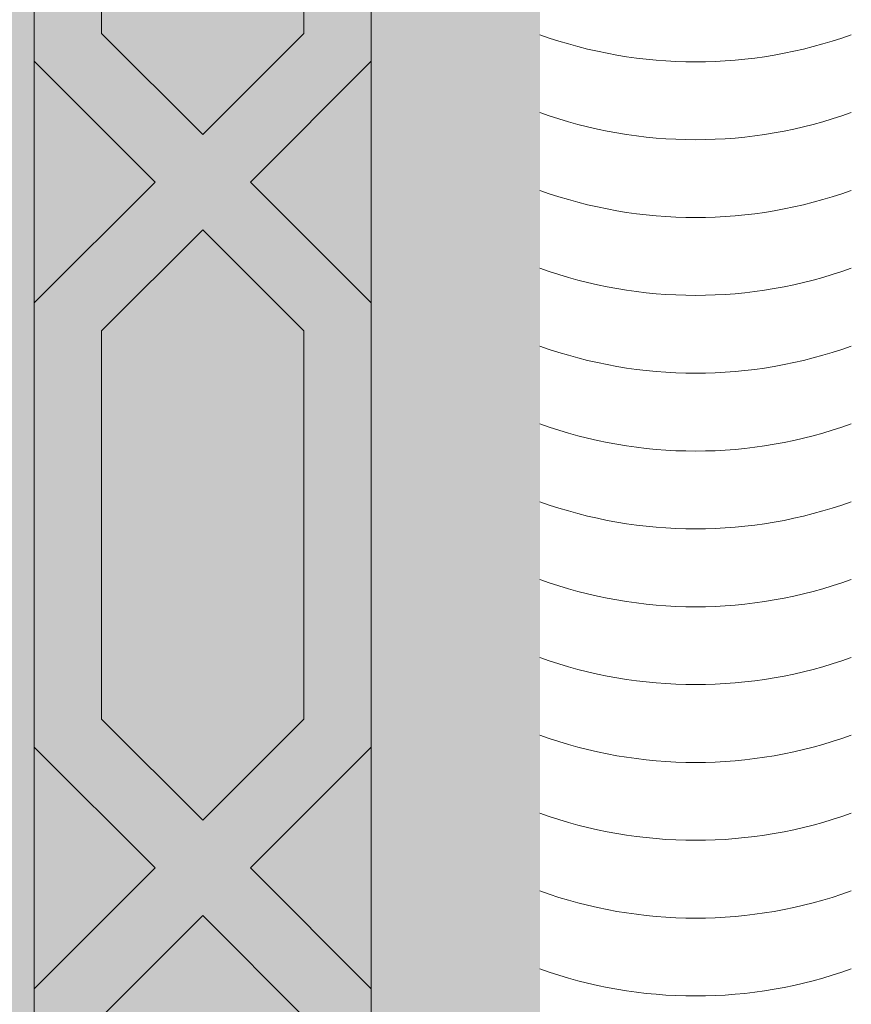
# Model space of a CAD drawing. Units: inches. Extents: x 844 to 2234, y 346 to 1084.
# Tile 39 of 93: x 1262.421 to 1265.567, y 701.353 to 705.079. Entities that reach past the tile are written whole.
import ezdxf

# ---------------------------------------------------------------- set-up
doc = ezdxf.new("R2010")
doc.units = ezdxf.units.IN
doc.header["$MEASUREMENT"] = 0
doc.layers.add('furniture', color=8, linetype='Continuous', lineweight=18)
doc.layers.add('RA-AP-01$0$INT', color=35, linetype='Continuous', lineweight=5)
doc.layers.add('RA-AP-01$0$FURN', color=3, linetype='Continuous')

# ---------------------------------------------------------------- blocks, each defined once
blk = doc.blocks.new('A$C18D01794')
at = {"layer": 'RA-AP-01$0$INT'}
h = blk.add_hatch(color=256, dxfattribs=at)
h.paths.add_polyline_path([(4.355206456958071, -6.156712009588037), (4.355206456958071, -8.056712009588038), (5.455206456958072, -8.056712009588038), (5.455206456958072, -6.156712009588037)])
h.paths.add_polyline_path([(4.405206456958072, -8.006712009588039), (4.405206456958072, -6.206712009588038), (5.405206456958072, -6.206712009588038), (5.405206456958072, -8.006712009588039)], flags=16)
h = blk.add_hatch(color=256, dxfattribs=at)
h.paths.add_polyline_path([(4.505206456958071, -7.585498806127123), (4.46934859260189, -7.549640941759413), (4.505206456958071, -7.513783077414768), (4.505206456958071, -7.381963272220687), (4.469348592616735, -7.346105407867824), (4.505206456958071, -7.310247543514964), (4.505206456958071, -7.178427738324996), (4.469348592586679, -7.142569873965138), (4.505206456952245, -7.106712009588038), (4.476922185709333, -7.106712009588038), (4.455206456960671, -7.128427738343681), (4.433490728198047, -7.106712009588038), (4.405206456946033, -7.106712009588036), (4.441064321339216, -7.142569873969684), (4.40520645695807, -7.178427738362358), (4.405206456958072, -7.310247543472698), (4.441064321364728, -7.346105407867826), (4.40520645695807, -7.381963272262947), (4.40520645695807, -7.513783077378263), (4.441064321354429, -7.549640941786153), (4.405206456958072, -7.585498806170974), (4.405206456958072, -7.717318611286652), (4.441064321333084, -7.753176475673194), (4.405206456958072, -7.789034340036673), (4.405206456958072, -8.006712009588039), (4.644348592588106, -8.006712009588039), (4.680206456964639, -7.970854145211967), (4.716064321341165, -8.006712009588039), (4.869348592586113, -8.006712009588039), (4.905206456964143, -7.970854145210465), (4.941064321342174, -8.006712009588039), (5.094348592587118, -8.006712009588037), (5.130206456963649, -7.970854145211967), (5.166064321340178, -8.006712009588039), (5.405206456958072, -8.006712009588039), (5.405206456958072, -7.789034340024526), (5.369348592595202, -7.753176475673196), (5.40520645695807, -7.717318611298797), (5.40520645695807, -7.585498806158829), (5.369348592573859, -7.549640941786151), (5.40520645695807, -7.51378307739041), (5.40520645695807, -7.381963272250803), (5.36934859256356, -7.346105407867824), (5.405206456958072, -7.310247543484846), (5.405206456958072, -7.178427738350217), (5.369348592589068, -7.142569873969682), (5.405206456982249, -7.106712009588038), (5.376922185730244, -7.106712009588038), (5.355206456967613, -7.128427738343679), (5.333490728218955, -7.10671200958804), (5.305206456976043, -7.106712009588042), (5.341064321341609, -7.142569873965136), (5.305206456958072, -7.178427738337141), (5.305206456958072, -7.310247543502816), (5.34106432131155, -7.346105407867824), (5.305206456958072, -7.381963272232832), (5.30520645695807, -7.513783077402624), (5.341064321326395, -7.549640941759413), (5.305206456958072, -7.585498806139263), (5.305206456958072, -7.717318611299605), (5.341064321347738, -7.753176475677737), (5.305206456958072, -7.78903434007894), (5.30520645695807, -7.906712009588039), (5.166064321336834, -7.906712009588039), (5.130206456963647, -7.942569873961684), (5.094348592590464, -7.906712009588039), (4.941064321338827, -7.906712009588041), (4.905206456964145, -7.942569873963183), (4.869348592589459, -7.906712009588039), (4.716064321337822, -7.906712009588041), (4.680206456964641, -7.942569873961684), (4.644348592591453, -7.906712009588039), (4.505206456958071, -7.906712009588039), (4.505206456958071, -7.789034340066795), (4.469348592580545, -7.753176475677738), (4.505206456958071, -7.717318611311748)])
h.paths.add_polyline_path([(4.485206456974132, -7.709034340046354), (4.45520645695909, -7.739034340051736), (4.425206456974128, -7.709034340057131), (4.425206456993394, -7.593783077384998), (4.45520645699153, -7.563783077396511), (4.485206456993396, -7.593783077408017)], flags=16)
h.paths.add_polyline_path([(4.455206456954537, -7.767318611299197), (4.485206456958242, -7.797318611312542), (4.48520645695951, -7.912569873958716), (4.45520645695415, -7.942569873954422), (4.425206456957888, -7.912569873967813), (4.425206456957888, -7.797318611286197)], flags=16)
h.paths.add_polyline_path([(4.455206456964794, -7.535498806149051), (4.42520645696469, -7.5054988061393), (4.425206456983954, -7.390247543486406), (4.455206456990734, -7.360247543489279), (4.485206456983953, -7.39024754349214), (4.485206456964687, -7.505498806158811)], flags=16)
h.paths.add_polyline_path([(4.499348592588947, -7.926712009585049), (4.636064321340932, -7.926712009585049), (4.666064321342317, -7.956712009586821), (4.636064321343707, -7.986712009585048), (4.499348592575121, -7.986712009585048), (4.469348592591685, -7.956712009591957)], flags=16)
h.paths.add_polyline_path([(4.425206456957888, -7.940854145195974), (4.471064321332215, -7.986712009585049), (4.425206456957888, -7.986712009585049)], flags=16)
h.paths.add_polyline_path([(4.455206456990734, -7.331963272246367), (4.425206456989053, -7.301963272254337), (4.425206456969784, -7.186712009596224), (4.455206456965226, -7.156712009591144), (4.485206456969787, -7.186712009586051), (4.485206456989053, -7.301963272238404)], flags=16)
h.paths.add_polyline_path([(4.72434859258714, -7.926712009586255), (4.861064321340141, -7.926712009586248), (4.891064321340324, -7.956712009586823), (4.861064321340513, -7.986712009586252), (4.724348592586768, -7.986712009586252), (4.694348592586956, -7.956712009586821)], flags=16)
h.paths.add_polyline_path([(4.919348592587961, -7.956712009586821), (4.949348592588145, -7.92671200958625), (5.08606432134115, -7.926712009586253), (5.116064321341327, -7.956712009586823), (5.086064321341519, -7.986712009586252), (4.949348592587774, -7.986712009586252)], flags=16)
h.paths.add_polyline_path([(5.144348592585967, -7.956712009586823), (5.174348592587358, -7.926712009585049), (5.311064321339338, -7.926712009585049), (5.3410643213366, -7.956712009591957), (5.311064321353163, -7.986712009585048), (5.174348592584576, -7.986712009585048)], flags=16)
h.paths.add_polyline_path([(5.32520645693489, -7.593783077408021), (5.355206456936755, -7.563783077396511), (5.385206456934894, -7.593783077384998), (5.38520645695416, -7.709034340057128), (5.355206456969194, -7.739034340051736), (5.325206456954153, -7.709034340046352)], flags=16)
h.paths.add_polyline_path([(5.325206456970042, -7.797318611312542), (5.355206456973747, -7.767318611299197), (5.385206456970398, -7.7973186112862), (5.385206456970398, -7.912569873967816), (5.355206456974136, -7.942569873954422), (5.325206456968778, -7.912569873958716)], flags=16)
h.paths.add_polyline_path([(5.325206456963599, -7.505498806158811), (5.325206456944333, -7.39024754349214), (5.355206456937552, -7.360247543489279), (5.385206456944332, -7.39024754348641), (5.385206456963596, -7.505498806139303), (5.355206456963492, -7.53549880614905)], flags=16)
h.paths.add_polyline_path([(5.32520645693923, -7.301963272238403), (5.3252064569585, -7.186712009586051), (5.355206456963062, -7.156712009591142), (5.3852064569585, -7.186712009596224), (5.385206456939234, -7.301963272254338), (5.355206456937552, -7.331963272246369)], flags=16)
h.paths.add_polyline_path([(5.339348592596071, -7.986712009585048), (5.385206456970398, -7.940854145195972), (5.385206456970396, -7.986712009585048)], flags=16)
h = blk.add_hatch(color=256, dxfattribs=at)
h.paths.add_polyline_path([(4.469348592586677, -7.142569873965136), (4.505206456958073, -7.178427738324996), (4.505206456958071, -7.106712009582215)])
h.paths.add_polyline_path([(4.455206456960671, -7.128427738343681), (4.476922185709333, -7.106712009588038), (4.433490728198045, -7.106712009588038)])
h.paths.add_polyline_path([(4.405206456958073, -7.178427738362358), (4.441064321339218, -7.142569873969684), (4.40520645695807, -7.106712009600073)])
h.paths.add_polyline_path([(4.425206456989053, -7.301963272254335), (4.455206456990736, -7.331963272246371), (4.485206456989055, -7.301963272238399), (4.48520645696979, -7.186712009586054), (4.455206456965227, -7.15671200959114), (4.425206456969784, -7.186712009596224)])
h.paths.add_polyline_path([(4.505206456958073, -7.381963272220689), (4.505206456958071, -7.310247543514961), (4.469348592616738, -7.346105407867826)])
h.paths.add_polyline_path([(4.425206456964688, -7.5054988061393), (4.455206456964794, -7.535498806149051), (4.485206456964689, -7.505498806158811), (4.485206456983951, -7.390247543492138), (4.455206456990736, -7.360247543489277), (4.425206456983956, -7.39024754348641)])
h.paths.add_polyline_path([(4.425206456974126, -7.709034340057128), (4.455206456959092, -7.739034340051736), (4.485206456974132, -7.709034340046356), (4.485206456993396, -7.593783077408017), (4.45520645699153, -7.563783077396511), (4.425206456993394, -7.593783077384999)])
h.paths.add_polyline_path([(4.46934859260189, -7.549640941759415), (4.505206456958071, -7.585498806127123), (4.505206456958073, -7.513783077414766)])
h.paths.add_polyline_path([(4.405206456958073, -7.585498806170972), (4.441064321354427, -7.549640941786151), (4.405206456958072, -7.513783077378263)])
h.paths.add_polyline_path([(4.405206456958072, -7.789034340036673), (4.441064321333084, -7.753176475673194), (4.405206456958072, -7.71731861128665)])
h.paths.add_polyline_path([(4.469348592580547, -7.75317647567774), (4.505206456958071, -7.789034340066795), (4.505206456958071, -7.717318611311744)])
h.paths.add_polyline_path([(4.425206456957888, -7.912569873967814), (4.45520645695415, -7.942569873954422), (4.485206456959507, -7.912569873958718), (4.48520645695824, -7.797318611312542), (4.455206456954537, -7.767318611299197), (4.425206456957888, -7.797318611286202)])
h.paths.add_polyline_path([(4.425206456957888, -7.986712009585049), (4.471064321332215, -7.986712009585049), (4.425206456957888, -7.940854145195972)])
h.paths.add_polyline_path([(4.499348592575121, -7.986712009585048), (4.636064321343707, -7.986712009585049), (4.666064321342317, -7.956712009586823), (4.636064321340932, -7.926712009585049), (4.499348592588945, -7.926712009585049), (4.469348592591685, -7.95671200959196)])
h.paths.add_polyline_path([(4.680206456964641, -7.942569873961684), (4.716064321337824, -7.906712009588039), (4.644348592591454, -7.906712009588039)])
h.paths.add_polyline_path([(4.644348592588108, -8.006712009588039), (4.716064321341167, -8.006712009588039), (4.680206456964637, -7.970854145211964)])
h.paths.add_polyline_path([(4.724348592586768, -7.98671200958625), (4.861064321340514, -7.986712009586252), (4.891064321340324, -7.956712009586819), (4.861064321340141, -7.92671200958625), (4.724348592587134, -7.926712009586255), (4.694348592586957, -7.956712009586821)])
h.paths.add_polyline_path([(4.905206456964143, -7.942569873963183), (4.941064321338827, -7.906712009588039), (4.869348592589457, -7.906712009588037)])
h.paths.add_polyline_path([(4.869348592586113, -8.006712009588039), (4.941064321342172, -8.006712009588037), (4.905206456964145, -7.970854145210463)])
h.paths.add_polyline_path([(4.949348592587774, -7.986712009586252), (5.086064321341521, -7.986712009586252), (5.116064321341329, -7.956712009586823), (5.08606432134115, -7.926712009586253), (4.949348592588145, -7.92671200958625), (4.919348592587961, -7.956712009586819)])
h.paths.add_polyline_path([(5.130206456963645, -7.942569873961684), (5.166064321336834, -7.906712009588039), (5.094348592590464, -7.906712009588039)])
h.paths.add_polyline_path([(5.094348592587119, -8.006712009588039), (5.166064321340178, -8.006712009588039), (5.130206456963651, -7.970854145211967)])
h.paths.add_polyline_path([(5.174348592584578, -7.986712009585048), (5.311064321353163, -7.986712009585048), (5.341064321336602, -7.956712009591958), (5.31106432133934, -7.926712009585049), (5.174348592587352, -7.926712009585049), (5.144348592585969, -7.956712009586823)])
h.paths.add_polyline_path([(5.325206456968778, -7.912569873958718), (5.355206456974136, -7.942569873954422), (5.385206456970396, -7.912569873967814), (5.385206456970396, -7.797318611286199), (5.355206456973747, -7.767318611299197), (5.325206456970044, -7.797318611312544)])
h.paths.add_polyline_path([(5.339348592596073, -7.986712009585048), (5.385206456970396, -7.986712009585049), (5.385206456970398, -7.94085414519597)])
h.paths.add_polyline_path([(5.325206456954155, -7.709034340046354), (5.355206456969194, -7.739034340051734), (5.38520645695416, -7.709034340057128), (5.385206456934896, -7.593783077384999), (5.355206456936758, -7.563783077396513), (5.325206456934888, -7.593783077408019)])
h.paths.add_polyline_path([(5.305206456958072, -7.789034340078938), (5.341064321347739, -7.753176475677738), (5.305206456958072, -7.717318611299605)])
h.paths.add_polyline_path([(5.369348592595204, -7.753176475673194), (5.40520645695807, -7.789034340024526), (5.405206456958072, -7.717318611298798)])
h.paths.add_polyline_path([(5.405206456958072, -7.585498806158831), (5.405206456958072, -7.513783077390407), (5.369348592573857, -7.549640941786151)])
h.paths.add_polyline_path([(5.305206456958072, -7.585498806139266), (5.341064321326393, -7.549640941759413), (5.305206456958072, -7.513783077402626)])
h.paths.add_polyline_path([(5.325206456963599, -7.50549880615881), (5.355206456963494, -7.535498806149055), (5.385206456963598, -7.505498806139302), (5.385206456944334, -7.390247543486411), (5.355206456937552, -7.360247543489279), (5.325206456944333, -7.39024754349214)])
h.paths.add_polyline_path([(5.305206456958072, -7.38196327223283), (5.341064321311551, -7.346105407867824), (5.305206456958072, -7.31024754350282)])
h.paths.add_polyline_path([(5.325206456939231, -7.301963272238404), (5.355206456937552, -7.331963272246369), (5.385206456939235, -7.301963272254335), (5.385206456958502, -7.186712009596224), (5.355206456963061, -7.156712009591142), (5.3252064569585, -7.186712009586051)])
h.paths.add_polyline_path([(5.404581768715993, -7.381338584008926, -0.001217816984214), (5.405206456958072, -7.381112009582329), (5.405206456958072, -7.310247543484846), (5.369348592563558, -7.346105407867826)])
h.paths.add_polyline_path([(5.36934859258907, -7.142569873969684), (5.40520645695807, -7.178427738350215), (5.405206456958072, -7.106712009612218)])
h.paths.add_polyline_path([(5.355206456967613, -7.128427738343683), (5.376922185730239, -7.106712009588038), (5.333490728218953, -7.10671200958804)])
h.paths.add_polyline_path([(5.30520645695807, -7.178427738337139), (5.341064321341609, -7.142569873965134), (5.305206456958074, -7.10671200957007)])
blk.add_hatch(color=256, dxfattribs=at).paths.add_polyline_path([(4.505206456958071, -7.906712009588039), (5.305206456958072, -7.906712009588039), (5.305206456958072, -7.106712009588038), (5.255206456951893, -7.106712009588036), (5.25520645694868, -7.856712009570104), (4.555206456959269, -7.856712009588616), (4.555206456956052, -7.106712009588038), (4.505206456958073, -7.106712009588038)])
for p, q in [((4.425206456964688, -7.5054988061393), (4.455206456964796, -7.535498806149051)), ((4.485206456964687, -7.505498806158811), (4.455206456964796, -7.535498806149051)), ((4.405206456968717, -7.513783077388909), (4.441064321338788, -7.54964094177051)), ((4.505206456968717, -7.513783077404122), (4.469348592586251, -7.549640941775054)), ((4.405206456988469, -7.585498806140577), (4.441064321370071, -7.549640941770508)), ((4.505206456988468, -7.58549880615752), (4.469348592617532, -7.549640941775056)), ((4.425206456993394, -7.593783077384996), (4.45520645699153, -7.563783077396511)), ((4.485206456993396, -7.593783077408017), (4.45520645699153, -7.563783077396511)), ((4.425206456993394, -7.593783077384996), (4.425206456974128, -7.709034340057129)), ((4.485206456993396, -7.593783077408017), (4.485206456974132, -7.709034340046354)), ((4.425206456974128, -7.709034340057129), (4.455206456959092, -7.739034340051736)), ((4.485206456974132, -7.709034340046354), (4.455206456959092, -7.739034340051736)), ((4.405206456963013, -7.717318611291593), (4.441064321333084, -7.753176475673194)), ((4.505206456963013, -7.717318611306806), (4.469348592580547, -7.753176475677738)), ((4.441064321333084, -7.753176475673194), (4.405206456950156, -7.789034340044587)), ((4.469348592580547, -7.753176475677738), (4.505206456951941, -7.789034340060664)), ((4.455206456954537, -7.767318611299197), (4.425206456957888, -7.797318611286199)), ((4.455206456954537, -7.767318611299197), (4.485206456958242, -7.797318611312544)), ((4.425206456957888, -7.797318611286199), (4.425206456957888, -7.912569873967814)), ((4.485206456959509, -7.912569873958718), (4.485206456958242, -7.797318611312544))]:
    blk.add_line(p, q, dxfattribs=at)
for points in [[(5.405206456958072, -8.006712009588039), (4.405206456958072, -8.006712009588039), (4.405206456958072, -7.106712009588038)], [(5.305206456958072, -7.106712009588038), (5.305206456958072, -7.906712009588039), (4.505206456958071, -7.906712009588039), (4.505206456958071, -7.106712009588038)]]:
    blk.add_lwpolyline(points, dxfattribs=at)
for centre in [(4.309006456954359, -7.648064458284158), (4.309006456951176, -7.671164458284799), (4.309006456954132, -7.671164458285863), (4.309006456953905, -7.694264458283548), (4.309006456953905, -7.717364458282297), (4.309006456952313, -7.740464458286957), (4.30900645695345, -7.763564458285706), (4.30900645695345, -7.786664458281272), (4.309006456951858, -7.80976445828616), (4.309006456950039, -7.832864458284682), (4.309006456952995, -7.855964458280475), (4.309006456952768, -7.879064458285135), (4.309006456951176, -7.902164458283884), (4.309006456949584, -7.925264458285589)]:
    blk.add_arc(centre, 0.136414042854523, 70.20384312815696, 109.7961568705686, dxfattribs=at)
blk = doc.blocks.new('A$C5D2F253E')
at = {"layer": 'RA-AP-01$0$FURN', "xscale": -0.7999999999883585, "yscale": 0.7999999999883585, "zscale": 0.8, "rotation": 90}
blk.add_blockref('A$C18D01794', (-5.687757199772477, 4.75791982714071), dxfattribs=at)

msp = doc.modelspace()

# ---------------------------------------------------------------- block references
at = {"layer": 'furniture', "xscale": -15.94108302203742, "yscale": 15.94108302203742, "zscale": 15.94108302203742, "rotation": 270}
msp.add_blockref('A$C5D2F253E', (1244.08405109492, 696.2584716700112), dxfattribs=at)

doc.saveas('drawing.dxf')
